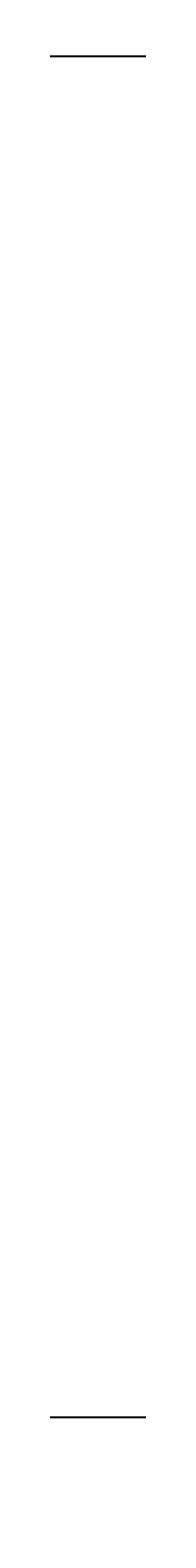
# Model space of a CAD drawing. Units: inches. Extents: x 35362 to 73946, y 43607 to 67532.
# Tile 20 of 134: x 48340 to 48365, y 46091 to 46564. Entities that reach past the tile are written whole.
import ezdxf

# ---------------------------------------------------------------- set-up
doc = ezdxf.new("R2010")
doc.units = ezdxf.units.IN
doc.header["$MEASUREMENT"] = 0
doc.layers.add('A-ANNO-DIMS', color=2, linetype='Continuous', lineweight=18)
doc.styles.get("Standard").update_dxf_attribs({"font": 'arial.ttf'})
doc.dimstyles.get("Standard").update_dxf_attribs({"dimtxt": 0.18, "dimasz": 0.18, "dimexe": 0.18, "dimexo": 0.0625, "dimgap": 0.09, "dimtad": 0, "dimtih": 1, "dimtoh": 1, "dimdec": 4, "dimzin": 0, "dimdsep": 46, "dimtxsty": 'Standard', "dimcen": 0.09, "dimadec": 0, "dimazin": 0, "dimtfac": 1, "dimtdec": 4, "dimtofl": 0, "dimtmove": 0, "dimatfit": 3, "dimfxl": 1, "dimtolj": 1, "dimtzin": 0, "dimarcsym": 0})

# ---------------------------------------------------------------- blocks, each defined once
blk = doc.blocks.new('*D5')
at = {"layer": 'A-ANNO-DIMS', "color": 0, "lineweight": -2, "transparency": 16777216}
for p, q in [((37121.95, 46919.32), (37121.95, 43606.68)), ((69871.5, 45449.83), (69871.5, 43606.68)), ((37122.13, 43606.86), (53496.29, 43606.86)), ((69871.32, 43606.86), (53497.15, 43606.86))]:
    blk.add_line(p, q, dxfattribs=at)
at = {"layer": 'A-ANNO-DIMS', "color": 0, "transparency": 16777216}
for points in [[(37122.13, 43606.89), (37122.13, 43606.83), (37121.95, 43606.86)], [(69871.32, 43606.89), (69871.32, 43606.83), (69871.5, 43606.86)]]:
    blk.add_solid(points, dxfattribs=at)
at = {"layer": 'Defpoints', "color": 0, "transparency": 16777216}
for p in [(37121.95, 46919.38), (69871.5, 45449.89), (69871.5, 43606.86)]:
    blk.add_point(p, dxfattribs=at)
at = {"layer": 'A-ANNO-DIMS', "color": 0, "transparency": 16777216, "insert": (53496.72, 43606.86), "char_height": 0.18, "attachment_point": 5}
blk.add_mtext('\\A1;32750', dxfattribs=at)
blk = doc.blocks.new('*D11')
at = {"layer": 'A-ANNO-DIMS', "color": 0, "lineweight": -2, "transparency": 16777216}
for p, q in [((47978.66, 56028.77), (47978.66, 43606.68)), ((53109.76, 56028.77), (53109.76, 43606.68)), ((47978.84, 43606.86), (50543.87, 43606.86)), ((53109.58, 43606.86), (50544.55, 43606.86))]:
    blk.add_line(p, q, dxfattribs=at)
at = {"layer": 'A-ANNO-DIMS', "color": 0, "transparency": 16777216}
for points in [[(47978.84, 43606.89), (47978.84, 43606.83), (47978.66, 43606.86)], [(53109.58, 43606.89), (53109.58, 43606.83), (53109.76, 43606.86)]]:
    blk.add_solid(points, dxfattribs=at)
at = {"layer": 'Defpoints', "color": 0, "transparency": 16777216}
for p in [(47978.66, 56028.84), (53109.76, 56028.84), (53109.76, 43606.86)]:
    blk.add_point(p, dxfattribs=at)
at = {"layer": 'A-ANNO-DIMS', "color": 0, "transparency": 16777216, "insert": (50544.21, 43606.86), "char_height": 0.18, "attachment_point": 5}
blk.add_mtext('\\A1;5131', dxfattribs=at)
blk = doc.blocks.new('*D27')
at = {"layer": 'A-ANNO-DIMS', "color": 0, "lineweight": -2, "transparency": 16777216}
for p, q in [((47978.66, 56028.77), (47978.66, 43606.68)), ((48373.49, 53428.96), (48373.49, 43606.68)), ((47978.84, 43606.86), (48175.68, 43606.86)), ((48373.31, 43606.86), (48176.47, 43606.86))]:
    blk.add_line(p, q, dxfattribs=at)
at = {"layer": 'A-ANNO-DIMS', "color": 0, "transparency": 16777216}
for points in [[(47978.84, 43606.89), (47978.84, 43606.83), (47978.66, 43606.86)], [(48373.31, 43606.89), (48373.31, 43606.83), (48373.49, 43606.86)]]:
    blk.add_solid(points, dxfattribs=at)
at = {"layer": 'Defpoints', "color": 0, "transparency": 16777216}
for p in [(47978.66, 56028.84), (48373.49, 53429.02), (48373.49, 43606.86)]:
    blk.add_point(p, dxfattribs=at)
at = {"layer": 'A-ANNO-DIMS', "color": 0, "transparency": 16777216, "insert": (48176.08, 43606.86), "char_height": 0.18, "attachment_point": 5}
blk.add_mtext('\\A1;394.8', dxfattribs=at)
blk = doc.blocks.new('*D67')
at = {"layer": 'A-ANNO-DIMS', "color": 0, "lineweight": -2, "transparency": 16777216}
for p, q in [((56873.54, 53351.53), (35361.77, 53351.53)), ((35361.95, 53351.35), (35361.95, 49400.89)), ((35361.95, 45450.07), (35361.95, 49400.53)), ((53793.58, 45449.89), (35361.77, 45449.89))]:
    blk.add_line(p, q, dxfattribs=at)
at = {"layer": 'A-ANNO-DIMS', "color": 0, "transparency": 16777216}
for points in [[(35361.92, 53351.35), (35361.98, 53351.35), (35361.95, 53351.53)], [(35361.92, 45450.07), (35361.98, 45450.07), (35361.95, 45449.89)]]:
    blk.add_solid(points, dxfattribs=at)
at = {"layer": 'Defpoints', "color": 0, "transparency": 16777216}
for p in [(35361.95, 53351.53), (56873.6, 53351.53), (53793.64, 45449.89)]:
    blk.add_point(p, dxfattribs=at)
at = {"layer": 'A-ANNO-DIMS', "color": 0, "transparency": 16777216, "insert": (35361.95, 49400.71), "char_height": 0.18, "attachment_point": 5}
blk.add_mtext('\\A1;7901.6', dxfattribs=at)
blk = doc.blocks.new('*D76')
at = {"layer": 'A-ANNO-DIMS', "color": 0, "lineweight": -2, "transparency": 16777216}
for p, q in [((54052.84, 46555.29), (35361.77, 46555.29)), ((35361.95, 46555.11), (35361.95, 46342.27)), ((35361.95, 46129.06), (35361.95, 46341.9)), ((53793.58, 46128.88), (35361.77, 46128.88))]:
    blk.add_line(p, q, dxfattribs=at)
at = {"layer": 'A-ANNO-DIMS', "color": 0, "transparency": 16777216}
for points in [[(35361.92, 46555.11), (35361.98, 46555.11), (35361.95, 46555.29)], [(35361.92, 46129.06), (35361.98, 46129.06), (35361.95, 46128.88)]]:
    blk.add_solid(points, dxfattribs=at)
at = {"layer": 'Defpoints', "color": 0, "transparency": 16777216}
for p in [(35361.95, 46555.29), (54052.9, 46555.29), (53793.64, 46128.88)]:
    blk.add_point(p, dxfattribs=at)
at = {"layer": 'A-ANNO-DIMS', "color": 0, "transparency": 16777216, "insert": (35361.95, 46342.09), "char_height": 0.18, "attachment_point": 5}
blk.add_mtext('\\A1;426.4', dxfattribs=at)
blk = doc.blocks.new('*D90')
at = {"layer": 'A-ANNO-DIMS', "color": 0, "lineweight": -2, "transparency": 16777216}
for p, q in [((53707.72, 47291.29), (35361.77, 47291.29)), ((35361.95, 47291.11), (35361.95, 46710.26)), ((35361.95, 46129.06), (35361.95, 46709.9)), ((53793.58, 46128.88), (35361.77, 46128.88))]:
    blk.add_line(p, q, dxfattribs=at)
at = {"layer": 'A-ANNO-DIMS', "color": 0, "transparency": 16777216}
for points in [[(35361.92, 47291.11), (35361.98, 47291.11), (35361.95, 47291.29)], [(35361.92, 46129.06), (35361.98, 46129.06), (35361.95, 46128.88)]]:
    blk.add_solid(points, dxfattribs=at)
at = {"layer": 'Defpoints', "color": 0, "transparency": 16777216}
for p in [(53707.78, 47291.29), (35361.95, 46128.88), (53793.64, 46128.88)]:
    blk.add_point(p, dxfattribs=at)
at = {"layer": 'A-ANNO-DIMS', "color": 0, "transparency": 16777216, "insert": (35361.95, 46710.08), "char_height": 0.18, "attachment_point": 5}
blk.add_mtext('\\A1;1162.4', dxfattribs=at)

msp = doc.modelspace()

# ---------------------------------------------------------------- dimensions: what is measured, and where the dimension line sits
at = {"layer": 'A-ANNO-DIMS'}
for base, p1, p2, override, picture, middle in [((53109.76, 43606.859), (47978.665, 56028.836), (53109.76, 56028.836), {"dimdec": 0, "dimlfac": 1, "dimrnd": 0, "dimzin": 0, "dimdsep": 46, "dimlunit": 2}, '*D11', (50544.212, 43606.859)), ((48373.492, 43606.859), (47978.665, 56028.836), (48373.492, 53429.019), {"dimdec": 1, "dimlfac": 1, "dimrnd": 0, "dimzin": 0, "dimdsep": 46, "dimlunit": 2}, '*D27', (48176.078, 43606.859)), ((69871.496, 43606.859), (37121.949, 46919.381), (69871.496, 45449.894), {"dimdec": 0, "dimlfac": 1, "dimrnd": 0, "dimzin": 0, "dimdsep": 46, "dimlunit": 2}, '*D5', (53496.723, 43606.859))]:
    dim = msp.add_linear_dim(base=base, p1=p1, p2=p2, dimstyle='Standard', override=override, dxfattribs=at)
    dim.commit()
    dim.dimension.update_dxf_attribs({"geometry": picture, "text_midpoint": middle})
for base, p1, p2, picture, middle in [((35361.949, 53351.529), (53793.638, 45449.894), (56873.602, 53351.529), '*D67', (35361.949, 49400.712)), ((35361.949, 46128.878), (53707.781, 47291.285), (53793.638, 46128.878), '*D90', (35361.949, 46710.081)), ((35361.949, 46555.293), (53793.638, 46128.878), (54052.899, 46555.293), '*D76', (35361.949, 46342.086))]:
    dim = msp.add_linear_dim(base=base, p1=p1, p2=p2, angle=90, dimstyle='Standard', override={"dimdec": 1, "dimlfac": 1, "dimrnd": 0, "dimzin": 0, "dimdsep": 46, "dimlunit": 2}, dxfattribs=at)
    dim.commit()
    dim.dimension.update_dxf_attribs({"geometry": picture, "text_midpoint": middle})

doc.saveas('drawing.dxf')
